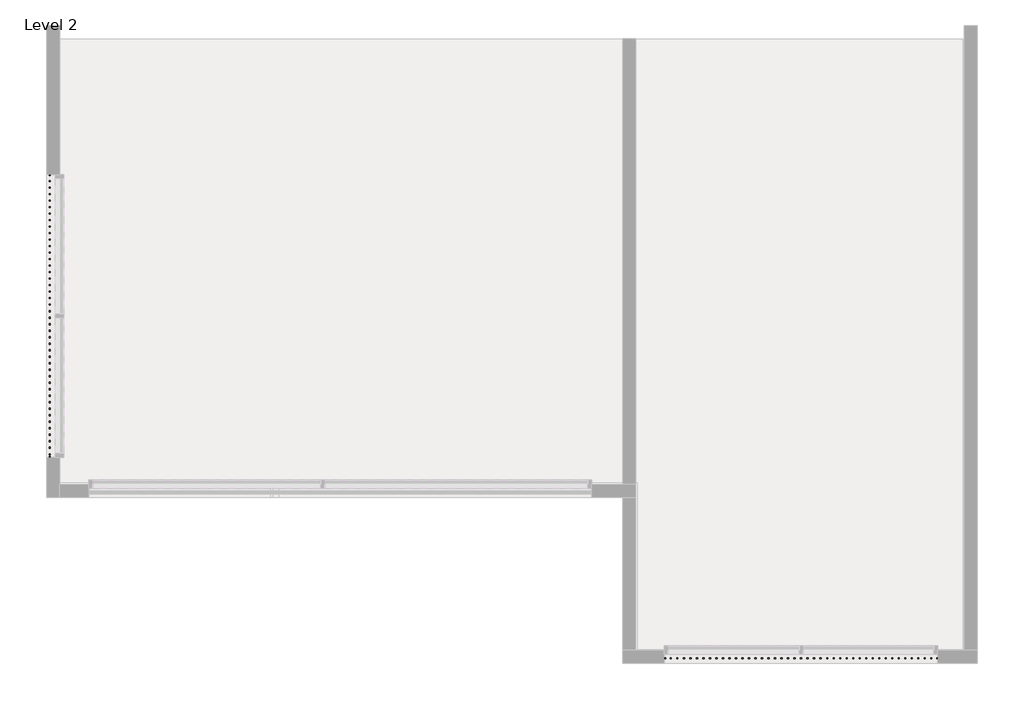
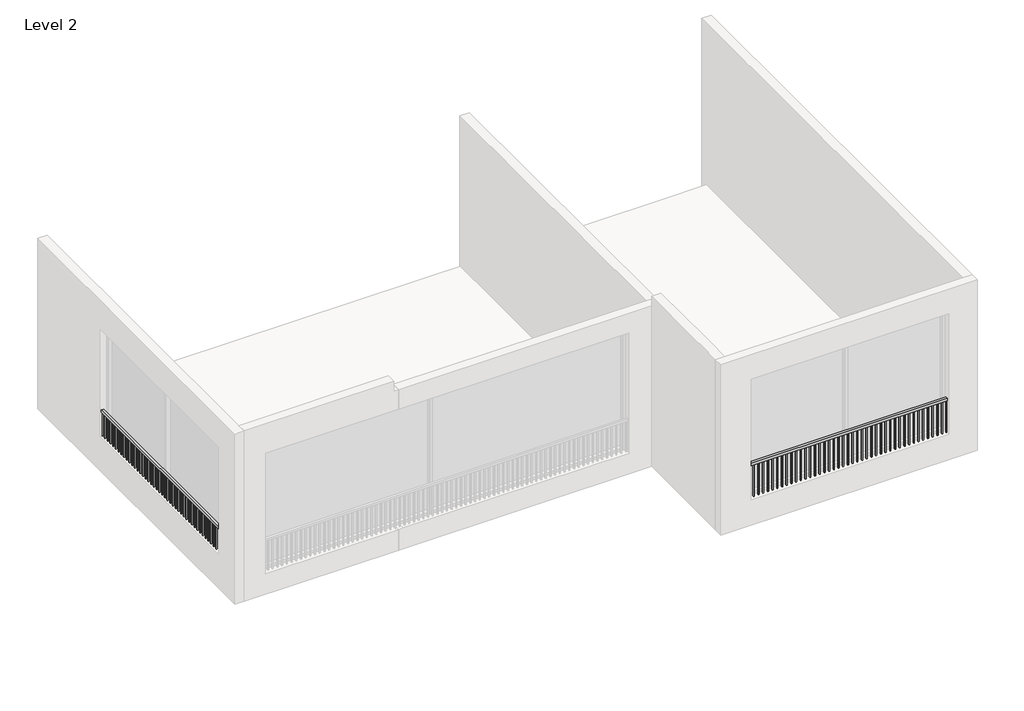
# One storey, part 2 of 2: 2 railings.
"""IFC4 building model written with IfcOpenShell, lengths in millimetres."""

from ifc_helpers import new_model, si_unit, frame, origin, place, context, project, spatial, polyline, outline, extrude, element, save

model = new_model("IFC4")

# Units and contexts
model_context = context("Model", 3, world=origin())
ifc_project = project(units=[si_unit("LENGTHUNIT", "METRE", prefix="MILLI")], contexts=[model_context])

# Site, building, storey
site = spatial("IfcSite", under=ifc_project)
building = spatial("IfcBuilding", under=site)
storey = spatial("IfcBuildingStorey", under=building, Name="Level 2", Elevation=3657.6)

# Railings
placement = place(None, origin())
element("IfcRailing", 1, ObjectType="Handrail - Rectangular", at=placement, inside=storey, context=model_context, shape_type="SweptSolid", body=[
    extrude(outline(polyline([(-6422.5796605, -2958.1874156), (-6422.5796605, -2907.3874156), (-2155.3796605, -2907.3874156), (-2155.3796605, -2958.1874156), (-6422.5796605, -2958.1874156)])), frame((0.0, 0.0, 4978.4), z_axis=(0.0, 0.0, 1.0), x_axis=(1.0, 0.0, 0.0)), (0.0, 0.0, 1.0), 50.8),
    extrude(outline(polyline([(-2266.5046605, -2942.3124156), (-2266.5046605, -2923.2624156), (-2247.4546605, -2923.2624156), (-2247.4546605, -2942.3124156), (-2266.5046605, -2942.3124156)])), frame((0.0, 0.0, 4114.8), z_axis=(0.0, 0.0, 1.0), x_axis=(1.0, 0.0, 0.0)), (0.0, 0.0, 1.0), 863.6),
    extrude(outline(polyline([(-2368.1046605, -2942.3124156), (-2368.1046605, -2923.2624156), (-2349.0546605, -2923.2624156), (-2349.0546605, -2942.3124156), (-2368.1046605, -2942.3124156)])), frame((0.0, 0.0, 4114.8), z_axis=(0.0, 0.0, 1.0), x_axis=(1.0, 0.0, 0.0)), (0.0, 0.0, 1.0), 863.6),
    extrude(outline(polyline([(-2469.7046605, -2942.3124156), (-2469.7046605, -2923.2624156), (-2450.6546605, -2923.2624156), (-2450.6546605, -2942.3124156), (-2469.7046605, -2942.3124156)])), frame((0.0, 0.0, 4114.8), z_axis=(0.0, 0.0, 1.0), x_axis=(1.0, 0.0, 0.0)), (0.0, 0.0, 1.0), 863.6),
    extrude(outline(polyline([(-2571.3046605, -2942.3124156), (-2571.3046605, -2923.2624156), (-2552.2546605, -2923.2624156), (-2552.2546605, -2942.3124156), (-2571.3046605, -2942.3124156)])), frame((0.0, 0.0, 4114.8), z_axis=(0.0, 0.0, 1.0), x_axis=(1.0, 0.0, 0.0)), (0.0, 0.0, 1.0), 863.6),
    extrude(outline(polyline([(-2672.9046605, -2942.3124156), (-2672.9046605, -2923.2624156), (-2653.8546605, -2923.2624156), (-2653.8546605, -2942.3124156), (-2672.9046605, -2942.3124156)])), frame((0.0, 0.0, 4114.8), z_axis=(0.0, 0.0, 1.0), x_axis=(1.0, 0.0, 0.0)), (0.0, 0.0, 1.0), 863.6),
    extrude(outline(polyline([(-2774.5046605, -2942.3124156), (-2774.5046605, -2923.2624156), (-2755.4546605, -2923.2624156), (-2755.4546605, -2942.3124156), (-2774.5046605, -2942.3124156)])), frame((0.0, 0.0, 4114.8), z_axis=(0.0, 0.0, 1.0), x_axis=(1.0, 0.0, 0.0)), (0.0, 0.0, 1.0), 863.6),
    extrude(outline(polyline([(-2876.1046605, -2942.3124156), (-2876.1046605, -2923.2624156), (-2857.0546605, -2923.2624156), (-2857.0546605, -2942.3124156), (-2876.1046605, -2942.3124156)])), frame((0.0, 0.0, 4114.8), z_axis=(0.0, 0.0, 1.0), x_axis=(1.0, 0.0, 0.0)), (0.0, 0.0, 1.0), 863.6),
    extrude(outline(polyline([(-2977.7046605, -2942.3124156), (-2977.7046605, -2923.2624156), (-2958.6546605, -2923.2624156), (-2958.6546605, -2942.3124156), (-2977.7046605, -2942.3124156)])), frame((0.0, 0.0, 4114.8), z_axis=(0.0, 0.0, 1.0), x_axis=(1.0, 0.0, 0.0)), (0.0, 0.0, 1.0), 863.6),
    extrude(outline(polyline([(-3079.3046605, -2942.3124156), (-3079.3046605, -2923.2624156), (-3060.2546605, -2923.2624156), (-3060.2546605, -2942.3124156), (-3079.3046605, -2942.3124156)])), frame((0.0, 0.0, 4114.8), z_axis=(0.0, 0.0, 1.0), x_axis=(1.0, 0.0, 0.0)), (0.0, 0.0, 1.0), 863.6),
    extrude(outline(polyline([(-3180.9046605, -2942.3124156), (-3180.9046605, -2923.2624156), (-3161.8546605, -2923.2624156), (-3161.8546605, -2942.3124156), (-3180.9046605, -2942.3124156)])), frame((0.0, 0.0, 4114.8), z_axis=(0.0, 0.0, 1.0), x_axis=(1.0, 0.0, 0.0)), (0.0, 0.0, 1.0), 863.6),
    extrude(outline(polyline([(-3282.5046605, -2942.3124156), (-3282.5046605, -2923.2624156), (-3263.4546605, -2923.2624156), (-3263.4546605, -2942.3124156), (-3282.5046605, -2942.3124156)])), frame((0.0, 0.0, 4114.8), z_axis=(0.0, 0.0, 1.0), x_axis=(1.0, 0.0, 0.0)), (0.0, 0.0, 1.0), 863.6),
    extrude(outline(polyline([(-3384.1046605, -2942.3124156), (-3384.1046605, -2923.2624156), (-3365.0546605, -2923.2624156), (-3365.0546605, -2942.3124156), (-3384.1046605, -2942.3124156)])), frame((0.0, 0.0, 4114.8), z_axis=(0.0, 0.0, 1.0), x_axis=(1.0, 0.0, 0.0)), (0.0, 0.0, 1.0), 863.6),
    extrude(outline(polyline([(-3485.7046605, -2942.3124156), (-3485.7046605, -2923.2624156), (-3466.6546605, -2923.2624156), (-3466.6546605, -2942.3124156), (-3485.7046605, -2942.3124156)])), frame((0.0, 0.0, 4114.8), z_axis=(0.0, 0.0, 1.0), x_axis=(1.0, 0.0, 0.0)), (0.0, 0.0, 1.0), 863.6),
    extrude(outline(polyline([(-3587.3046605, -2942.3124156), (-3587.3046605, -2923.2624156), (-3568.2546605, -2923.2624156), (-3568.2546605, -2942.3124156), (-3587.3046605, -2942.3124156)])), frame((0.0, 0.0, 4114.8), z_axis=(0.0, 0.0, 1.0), x_axis=(1.0, 0.0, 0.0)), (0.0, 0.0, 1.0), 863.6),
    extrude(outline(polyline([(-3688.9046605, -2942.3124156), (-3688.9046605, -2923.2624156), (-3669.8546605, -2923.2624156), (-3669.8546605, -2942.3124156), (-3688.9046605, -2942.3124156)])), frame((0.0, 0.0, 4114.8), z_axis=(0.0, 0.0, 1.0), x_axis=(1.0, 0.0, 0.0)), (0.0, 0.0, 1.0), 863.6),
    extrude(outline(polyline([(-3790.5046605, -2942.3124156), (-3790.5046605, -2923.2624156), (-3771.4546605, -2923.2624156), (-3771.4546605, -2942.3124156), (-3790.5046605, -2942.3124156)])), frame((0.0, 0.0, 4114.8), z_axis=(0.0, 0.0, 1.0), x_axis=(1.0, 0.0, 0.0)), (0.0, 0.0, 1.0), 863.6),
    extrude(outline(polyline([(-3892.1046605, -2942.3124156), (-3892.1046605, -2923.2624156), (-3873.0546605, -2923.2624156), (-3873.0546605, -2942.3124156), (-3892.1046605, -2942.3124156)])), frame((0.0, 0.0, 4114.8), z_axis=(0.0, 0.0, 1.0), x_axis=(1.0, 0.0, 0.0)), (0.0, 0.0, 1.0), 863.6),
    extrude(outline(polyline([(-3993.7046605, -2942.3124156), (-3993.7046605, -2923.2624156), (-3974.6546605, -2923.2624156), (-3974.6546605, -2942.3124156), (-3993.7046605, -2942.3124156)])), frame((0.0, 0.0, 4114.8), z_axis=(0.0, 0.0, 1.0), x_axis=(1.0, 0.0, 0.0)), (0.0, 0.0, 1.0), 863.6),
    extrude(outline(polyline([(-4095.3046605, -2942.3124156), (-4095.3046605, -2923.2624156), (-4076.2546605, -2923.2624156), (-4076.2546605, -2942.3124156), (-4095.3046605, -2942.3124156)])), frame((0.0, 0.0, 4114.8), z_axis=(0.0, 0.0, 1.0), x_axis=(1.0, 0.0, 0.0)), (0.0, 0.0, 1.0), 863.6),
    extrude(outline(polyline([(-4196.9046605, -2942.3124156), (-4196.9046605, -2923.2624156), (-4177.8546605, -2923.2624156), (-4177.8546605, -2942.3124156), (-4196.9046605, -2942.3124156)])), frame((0.0, 0.0, 4114.8), z_axis=(0.0, 0.0, 1.0), x_axis=(1.0, 0.0, 0.0)), (0.0, 0.0, 1.0), 863.6),
    extrude(outline(polyline([(-4298.5046605, -2942.3124156), (-4298.5046605, -2923.2624156), (-4279.4546605, -2923.2624156), (-4279.4546605, -2942.3124156), (-4298.5046605, -2942.3124156)])), frame((0.0, 0.0, 4114.8), z_axis=(0.0, 0.0, 1.0), x_axis=(1.0, 0.0, 0.0)), (0.0, 0.0, 1.0), 863.6),
    extrude(outline(polyline([(-4400.1046605, -2942.3124156), (-4400.1046605, -2923.2624156), (-4381.0546605, -2923.2624156), (-4381.0546605, -2942.3124156), (-4400.1046605, -2942.3124156)])), frame((0.0, 0.0, 4114.8), z_axis=(0.0, 0.0, 1.0), x_axis=(1.0, 0.0, 0.0)), (0.0, 0.0, 1.0), 863.6),
    extrude(outline(polyline([(-4501.7046605, -2942.3124156), (-4501.7046605, -2923.2624156), (-4482.6546605, -2923.2624156), (-4482.6546605, -2942.3124156), (-4501.7046605, -2942.3124156)])), frame((0.0, 0.0, 4114.8), z_axis=(0.0, 0.0, 1.0), x_axis=(1.0, 0.0, 0.0)), (0.0, 0.0, 1.0), 863.6),
    extrude(outline(polyline([(-4603.3046605, -2942.3124156), (-4603.3046605, -2923.2624156), (-4584.2546605, -2923.2624156), (-4584.2546605, -2942.3124156), (-4603.3046605, -2942.3124156)])), frame((0.0, 0.0, 4114.8), z_axis=(0.0, 0.0, 1.0), x_axis=(1.0, 0.0, 0.0)), (0.0, 0.0, 1.0), 863.6),
    extrude(outline(polyline([(-4704.9046605, -2942.3124156), (-4704.9046605, -2923.2624156), (-4685.8546605, -2923.2624156), (-4685.8546605, -2942.3124156), (-4704.9046605, -2942.3124156)])), frame((0.0, 0.0, 4114.8), z_axis=(0.0, 0.0, 1.0), x_axis=(1.0, 0.0, 0.0)), (0.0, 0.0, 1.0), 863.6),
    extrude(outline(polyline([(-4806.5046605, -2942.3124156), (-4806.5046605, -2923.2624156), (-4787.4546605, -2923.2624156), (-4787.4546605, -2942.3124156), (-4806.5046605, -2942.3124156)])), frame((0.0, 0.0, 4114.8), z_axis=(0.0, 0.0, 1.0), x_axis=(1.0, 0.0, 0.0)), (0.0, 0.0, 1.0), 863.6),
    extrude(outline(polyline([(-4908.1046605, -2942.3124156), (-4908.1046605, -2923.2624156), (-4889.0546605, -2923.2624156), (-4889.0546605, -2942.3124156), (-4908.1046605, -2942.3124156)])), frame((0.0, 0.0, 4114.8), z_axis=(0.0, 0.0, 1.0), x_axis=(1.0, 0.0, 0.0)), (0.0, 0.0, 1.0), 863.6),
    extrude(outline(polyline([(-5009.7046605, -2942.3124156), (-5009.7046605, -2923.2624156), (-4990.6546605, -2923.2624156), (-4990.6546605, -2942.3124156), (-5009.7046605, -2942.3124156)])), frame((0.0, 0.0, 4114.8), z_axis=(0.0, 0.0, 1.0), x_axis=(1.0, 0.0, 0.0)), (0.0, 0.0, 1.0), 863.6),
    extrude(outline(polyline([(-5111.3046605, -2942.3124156), (-5111.3046605, -2923.2624156), (-5092.2546605, -2923.2624156), (-5092.2546605, -2942.3124156), (-5111.3046605, -2942.3124156)])), frame((0.0, 0.0, 4114.8), z_axis=(0.0, 0.0, 1.0), x_axis=(1.0, 0.0, 0.0)), (0.0, 0.0, 1.0), 863.6),
    extrude(outline(polyline([(-5212.9046605, -2942.3124156), (-5212.9046605, -2923.2624156), (-5193.8546605, -2923.2624156), (-5193.8546605, -2942.3124156), (-5212.9046605, -2942.3124156)])), frame((0.0, 0.0, 4114.8), z_axis=(0.0, 0.0, 1.0), x_axis=(1.0, 0.0, 0.0)), (0.0, 0.0, 1.0), 863.6),
    extrude(outline(polyline([(-5314.5046605, -2942.3124156), (-5314.5046605, -2923.2624156), (-5295.4546605, -2923.2624156), (-5295.4546605, -2942.3124156), (-5314.5046605, -2942.3124156)])), frame((0.0, 0.0, 4114.8), z_axis=(0.0, 0.0, 1.0), x_axis=(1.0, 0.0, 0.0)), (0.0, 0.0, 1.0), 863.6),
    extrude(outline(polyline([(-5416.1046605, -2942.3124156), (-5416.1046605, -2923.2624156), (-5397.0546605, -2923.2624156), (-5397.0546605, -2942.3124156), (-5416.1046605, -2942.3124156)])), frame((0.0, 0.0, 4114.8), z_axis=(0.0, 0.0, 1.0), x_axis=(1.0, 0.0, 0.0)), (0.0, 0.0, 1.0), 863.6),
    extrude(outline(polyline([(-5517.7046605, -2942.3124156), (-5517.7046605, -2923.2624156), (-5498.6546605, -2923.2624156), (-5498.6546605, -2942.3124156), (-5517.7046605, -2942.3124156)])), frame((0.0, 0.0, 4114.8), z_axis=(0.0, 0.0, 1.0), x_axis=(1.0, 0.0, 0.0)), (0.0, 0.0, 1.0), 863.6),
    extrude(outline(polyline([(-5619.3046605, -2942.3124156), (-5619.3046605, -2923.2624156), (-5600.2546605, -2923.2624156), (-5600.2546605, -2942.3124156), (-5619.3046605, -2942.3124156)])), frame((0.0, 0.0, 4114.8), z_axis=(0.0, 0.0, 1.0), x_axis=(1.0, 0.0, 0.0)), (0.0, 0.0, 1.0), 863.6),
    extrude(outline(polyline([(-5720.9046605, -2942.3124156), (-5720.9046605, -2923.2624156), (-5701.8546605, -2923.2624156), (-5701.8546605, -2942.3124156), (-5720.9046605, -2942.3124156)])), frame((0.0, 0.0, 4114.8), z_axis=(0.0, 0.0, 1.0), x_axis=(1.0, 0.0, 0.0)), (0.0, 0.0, 1.0), 863.6),
    extrude(outline(polyline([(-5822.5046605, -2942.3124156), (-5822.5046605, -2923.2624156), (-5803.4546605, -2923.2624156), (-5803.4546605, -2942.3124156), (-5822.5046605, -2942.3124156)])), frame((0.0, 0.0, 4114.8), z_axis=(0.0, 0.0, 1.0), x_axis=(1.0, 0.0, 0.0)), (0.0, 0.0, 1.0), 863.6),
    extrude(outline(polyline([(-5924.1046605, -2942.3124156), (-5924.1046605, -2923.2624156), (-5905.0546605, -2923.2624156), (-5905.0546605, -2942.3124156), (-5924.1046605, -2942.3124156)])), frame((0.0, 0.0, 4114.8), z_axis=(0.0, 0.0, 1.0), x_axis=(1.0, 0.0, 0.0)), (0.0, 0.0, 1.0), 863.6),
    extrude(outline(polyline([(-6025.7046605, -2942.3124156), (-6025.7046605, -2923.2624156), (-6006.6546605, -2923.2624156), (-6006.6546605, -2942.3124156), (-6025.7046605, -2942.3124156)])), frame((0.0, 0.0, 4114.8), z_axis=(0.0, 0.0, 1.0), x_axis=(1.0, 0.0, 0.0)), (0.0, 0.0, 1.0), 863.6),
    extrude(outline(polyline([(-6127.3046605, -2942.3124156), (-6127.3046605, -2923.2624156), (-6108.2546605, -2923.2624156), (-6108.2546605, -2942.3124156), (-6127.3046605, -2942.3124156)])), frame((0.0, 0.0, 4114.8), z_axis=(0.0, 0.0, 1.0), x_axis=(1.0, 0.0, 0.0)), (0.0, 0.0, 1.0), 863.6),
    extrude(outline(polyline([(-6228.9046605, -2942.3124156), (-6228.9046605, -2923.2624156), (-6209.8546605, -2923.2624156), (-6209.8546605, -2942.3124156), (-6228.9046605, -2942.3124156)])), frame((0.0, 0.0, 4114.8), z_axis=(0.0, 0.0, 1.0), x_axis=(1.0, 0.0, 0.0)), (0.0, 0.0, 1.0), 863.6),
    extrude(outline(polyline([(-6330.5046605, -2942.3124156), (-6330.5046605, -2923.2624156), (-6311.4546605, -2923.2624156), (-6311.4546605, -2942.3124156), (-6330.5046605, -2942.3124156)])), frame((0.0, 0.0, 4114.8), z_axis=(0.0, 0.0, 1.0), x_axis=(1.0, 0.0, 0.0)), (0.0, 0.0, 1.0), 863.6),
    extrude(outline(polyline([(-2174.4296605, -2942.3124156), (-2174.4296605, -2923.2624156), (-2155.3796605, -2923.2624156), (-2155.3796605, -2942.3124156), (-2174.4296605, -2942.3124156)])), frame((0.0, 0.0, 4114.8), z_axis=(0.0, 0.0, 1.0), x_axis=(1.0, 0.0, 0.0)), (0.0, 0.0, 1.0), 863.6),
    extrude(outline(polyline([(-6422.5796605, -2942.3124156), (-6422.5796605, -2923.2624156), (-6403.5296605, -2923.2624156), (-6403.5296605, -2942.3124156), (-6422.5796605, -2942.3124156)])), frame((0.0, 0.0, 4114.8), z_axis=(0.0, 0.0, 1.0), x_axis=(1.0, 0.0, 0.0)), (0.0, 0.0, 1.0), 863.6),
])
element("IfcRailing", 2, ObjectType="Handrail - Rectangular", at=placement, inside=storey, context=model_context, shape_type="SweptSolid", body=[
    extrude(outline(polyline([(-16039.6141623, 4621.1544753), (-15988.8141623, 4621.1544753), (-15988.8141623, 201.5544753), (-16039.6141623, 201.5544753), (-16039.6141623, 4621.1544753)])), frame((0.0, 0.0, 4978.4), z_axis=(0.0, 0.0, 1.0), x_axis=(1.0, 0.0, 0.0)), (0.0, 0.0, 1.0), 50.8),
    extrude(outline(polyline([(-16023.7391623, 261.8794753), (-16004.6891623, 261.8794753), (-16004.6891623, 242.8294753), (-16023.7391623, 242.8294753), (-16023.7391623, 261.8794753)])), frame((0.0, 0.0, 4114.8), z_axis=(0.0, 0.0, 1.0), x_axis=(1.0, 0.0, 0.0)), (0.0, 0.0, 1.0), 863.6),
    extrude(outline(polyline([(-16023.7391623, 363.4794753), (-16004.6891623, 363.4794753), (-16004.6891623, 344.4294753), (-16023.7391623, 344.4294753), (-16023.7391623, 363.4794753)])), frame((0.0, 0.0, 4114.8), z_axis=(0.0, 0.0, 1.0), x_axis=(1.0, 0.0, 0.0)), (0.0, 0.0, 1.0), 863.6),
    extrude(outline(polyline([(-16023.7391623, 465.0794753), (-16004.6891623, 465.0794753), (-16004.6891623, 446.0294753), (-16023.7391623, 446.0294753), (-16023.7391623, 465.0794753)])), frame((0.0, 0.0, 4114.8), z_axis=(0.0, 0.0, 1.0), x_axis=(1.0, 0.0, 0.0)), (0.0, 0.0, 1.0), 863.6),
    extrude(outline(polyline([(-16023.7391623, 566.6794753), (-16004.6891623, 566.6794753), (-16004.6891623, 547.6294753), (-16023.7391623, 547.6294753), (-16023.7391623, 566.6794753)])), frame((0.0, 0.0, 4114.8), z_axis=(0.0, 0.0, 1.0), x_axis=(1.0, 0.0, 0.0)), (0.0, 0.0, 1.0), 863.6),
    extrude(outline(polyline([(-16023.7391623, 668.2794753), (-16004.6891623, 668.2794753), (-16004.6891623, 649.2294753), (-16023.7391623, 649.2294753), (-16023.7391623, 668.2794753)])), frame((0.0, 0.0, 4114.8), z_axis=(0.0, 0.0, 1.0), x_axis=(1.0, 0.0, 0.0)), (0.0, 0.0, 1.0), 863.6),
    extrude(outline(polyline([(-16023.7391623, 769.8794753), (-16004.6891623, 769.8794753), (-16004.6891623, 750.8294753), (-16023.7391623, 750.8294753), (-16023.7391623, 769.8794753)])), frame((0.0, 0.0, 4114.8), z_axis=(0.0, 0.0, 1.0), x_axis=(1.0, 0.0, 0.0)), (0.0, 0.0, 1.0), 863.6),
    extrude(outline(polyline([(-16023.7391623, 871.4794753), (-16004.6891623, 871.4794753), (-16004.6891623, 852.4294753), (-16023.7391623, 852.4294753), (-16023.7391623, 871.4794753)])), frame((0.0, 0.0, 4114.8), z_axis=(0.0, 0.0, 1.0), x_axis=(1.0, 0.0, 0.0)), (0.0, 0.0, 1.0), 863.6),
    extrude(outline(polyline([(-16023.7391623, 973.0794753), (-16004.6891623, 973.0794753), (-16004.6891623, 954.0294753), (-16023.7391623, 954.0294753), (-16023.7391623, 973.0794753)])), frame((0.0, 0.0, 4114.8), z_axis=(0.0, 0.0, 1.0), x_axis=(1.0, 0.0, 0.0)), (0.0, 0.0, 1.0), 863.6),
    extrude(outline(polyline([(-16023.7391623, 1074.6794753), (-16004.6891623, 1074.6794753), (-16004.6891623, 1055.6294753), (-16023.7391623, 1055.6294753), (-16023.7391623, 1074.6794753)])), frame((0.0, 0.0, 4114.8), z_axis=(0.0, 0.0, 1.0), x_axis=(1.0, 0.0, 0.0)), (0.0, 0.0, 1.0), 863.6),
    extrude(outline(polyline([(-16023.7391623, 1176.2794753), (-16004.6891623, 1176.2794753), (-16004.6891623, 1157.2294753), (-16023.7391623, 1157.2294753), (-16023.7391623, 1176.2794753)])), frame((0.0, 0.0, 4114.8), z_axis=(0.0, 0.0, 1.0), x_axis=(1.0, 0.0, 0.0)), (0.0, 0.0, 1.0), 863.6),
    extrude(outline(polyline([(-16023.7391623, 1277.8794753), (-16004.6891623, 1277.8794753), (-16004.6891623, 1258.8294753), (-16023.7391623, 1258.8294753), (-16023.7391623, 1277.8794753)])), frame((0.0, 0.0, 4114.8), z_axis=(0.0, 0.0, 1.0), x_axis=(1.0, 0.0, 0.0)), (0.0, 0.0, 1.0), 863.6),
    extrude(outline(polyline([(-16023.7391623, 1379.4794753), (-16004.6891623, 1379.4794753), (-16004.6891623, 1360.4294753), (-16023.7391623, 1360.4294753), (-16023.7391623, 1379.4794753)])), frame((0.0, 0.0, 4114.8), z_axis=(0.0, 0.0, 1.0), x_axis=(1.0, 0.0, 0.0)), (0.0, 0.0, 1.0), 863.6),
    extrude(outline(polyline([(-16023.7391623, 1481.0794753), (-16004.6891623, 1481.0794753), (-16004.6891623, 1462.0294753), (-16023.7391623, 1462.0294753), (-16023.7391623, 1481.0794753)])), frame((0.0, 0.0, 4114.8), z_axis=(0.0, 0.0, 1.0), x_axis=(1.0, 0.0, 0.0)), (0.0, 0.0, 1.0), 863.6),
    extrude(outline(polyline([(-16023.7391623, 1582.6794753), (-16004.6891623, 1582.6794753), (-16004.6891623, 1563.6294753), (-16023.7391623, 1563.6294753), (-16023.7391623, 1582.6794753)])), frame((0.0, 0.0, 4114.8), z_axis=(0.0, 0.0, 1.0), x_axis=(1.0, 0.0, 0.0)), (0.0, 0.0, 1.0), 863.6),
    extrude(outline(polyline([(-16023.7391623, 1684.2794753), (-16004.6891623, 1684.2794753), (-16004.6891623, 1665.2294753), (-16023.7391623, 1665.2294753), (-16023.7391623, 1684.2794753)])), frame((0.0, 0.0, 4114.8), z_axis=(0.0, 0.0, 1.0), x_axis=(1.0, 0.0, 0.0)), (0.0, 0.0, 1.0), 863.6),
    extrude(outline(polyline([(-16023.7391623, 1785.8794753), (-16004.6891623, 1785.8794753), (-16004.6891623, 1766.8294753), (-16023.7391623, 1766.8294753), (-16023.7391623, 1785.8794753)])), frame((0.0, 0.0, 4114.8), z_axis=(0.0, 0.0, 1.0), x_axis=(1.0, 0.0, 0.0)), (0.0, 0.0, 1.0), 863.6),
    extrude(outline(polyline([(-16023.7391623, 1887.4794753), (-16004.6891623, 1887.4794753), (-16004.6891623, 1868.4294753), (-16023.7391623, 1868.4294753), (-16023.7391623, 1887.4794753)])), frame((0.0, 0.0, 4114.8), z_axis=(0.0, 0.0, 1.0), x_axis=(1.0, 0.0, 0.0)), (0.0, 0.0, 1.0), 863.6),
    extrude(outline(polyline([(-16023.7391623, 1989.0794753), (-16004.6891623, 1989.0794753), (-16004.6891623, 1970.0294753), (-16023.7391623, 1970.0294753), (-16023.7391623, 1989.0794753)])), frame((0.0, 0.0, 4114.8), z_axis=(0.0, 0.0, 1.0), x_axis=(1.0, 0.0, 0.0)), (0.0, 0.0, 1.0), 863.6),
    extrude(outline(polyline([(-16023.7391623, 2090.6794753), (-16004.6891623, 2090.6794753), (-16004.6891623, 2071.6294753), (-16023.7391623, 2071.6294753), (-16023.7391623, 2090.6794753)])), frame((0.0, 0.0, 4114.8), z_axis=(0.0, 0.0, 1.0), x_axis=(1.0, 0.0, 0.0)), (0.0, 0.0, 1.0), 863.6),
    extrude(outline(polyline([(-16023.7391623, 2192.2794753), (-16004.6891623, 2192.2794753), (-16004.6891623, 2173.2294753), (-16023.7391623, 2173.2294753), (-16023.7391623, 2192.2794753)])), frame((0.0, 0.0, 4114.8), z_axis=(0.0, 0.0, 1.0), x_axis=(1.0, 0.0, 0.0)), (0.0, 0.0, 1.0), 863.6),
    extrude(outline(polyline([(-16023.7391623, 2293.8794753), (-16004.6891623, 2293.8794753), (-16004.6891623, 2274.8294753), (-16023.7391623, 2274.8294753), (-16023.7391623, 2293.8794753)])), frame((0.0, 0.0, 4114.8), z_axis=(0.0, 0.0, 1.0), x_axis=(1.0, 0.0, 0.0)), (0.0, 0.0, 1.0), 863.6),
    extrude(outline(polyline([(-16023.7391623, 2395.4794753), (-16004.6891623, 2395.4794753), (-16004.6891623, 2376.4294753), (-16023.7391623, 2376.4294753), (-16023.7391623, 2395.4794753)])), frame((0.0, 0.0, 4114.8), z_axis=(0.0, 0.0, 1.0), x_axis=(1.0, 0.0, 0.0)), (0.0, 0.0, 1.0), 863.6),
    extrude(outline(polyline([(-16023.7391623, 2497.0794753), (-16004.6891623, 2497.0794753), (-16004.6891623, 2478.0294753), (-16023.7391623, 2478.0294753), (-16023.7391623, 2497.0794753)])), frame((0.0, 0.0, 4114.8), z_axis=(0.0, 0.0, 1.0), x_axis=(1.0, 0.0, 0.0)), (0.0, 0.0, 1.0), 863.6),
    extrude(outline(polyline([(-16023.7391623, 2598.6794753), (-16004.6891623, 2598.6794753), (-16004.6891623, 2579.6294753), (-16023.7391623, 2579.6294753), (-16023.7391623, 2598.6794753)])), frame((0.0, 0.0, 4114.8), z_axis=(0.0, 0.0, 1.0), x_axis=(1.0, 0.0, 0.0)), (0.0, 0.0, 1.0), 863.6),
    extrude(outline(polyline([(-16023.7391623, 2700.2794753), (-16004.6891623, 2700.2794753), (-16004.6891623, 2681.2294753), (-16023.7391623, 2681.2294753), (-16023.7391623, 2700.2794753)])), frame((0.0, 0.0, 4114.8), z_axis=(0.0, 0.0, 1.0), x_axis=(1.0, 0.0, 0.0)), (0.0, 0.0, 1.0), 863.6),
    extrude(outline(polyline([(-16023.7391623, 2801.8794753), (-16004.6891623, 2801.8794753), (-16004.6891623, 2782.8294753), (-16023.7391623, 2782.8294753), (-16023.7391623, 2801.8794753)])), frame((0.0, 0.0, 4114.8), z_axis=(0.0, 0.0, 1.0), x_axis=(1.0, 0.0, 0.0)), (0.0, 0.0, 1.0), 863.6),
    extrude(outline(polyline([(-16023.7391623, 2903.4794753), (-16004.6891623, 2903.4794753), (-16004.6891623, 2884.4294753), (-16023.7391623, 2884.4294753), (-16023.7391623, 2903.4794753)])), frame((0.0, 0.0, 4114.8), z_axis=(0.0, 0.0, 1.0), x_axis=(1.0, 0.0, 0.0)), (0.0, 0.0, 1.0), 863.6),
    extrude(outline(polyline([(-16023.7391623, 3005.0794753), (-16004.6891623, 3005.0794753), (-16004.6891623, 2986.0294753), (-16023.7391623, 2986.0294753), (-16023.7391623, 3005.0794753)])), frame((0.0, 0.0, 4114.8), z_axis=(0.0, 0.0, 1.0), x_axis=(1.0, 0.0, 0.0)), (0.0, 0.0, 1.0), 863.6),
    extrude(outline(polyline([(-16023.7391623, 3106.6794753), (-16004.6891623, 3106.6794753), (-16004.6891623, 3087.6294753), (-16023.7391623, 3087.6294753), (-16023.7391623, 3106.6794753)])), frame((0.0, 0.0, 4114.8), z_axis=(0.0, 0.0, 1.0), x_axis=(1.0, 0.0, 0.0)), (0.0, 0.0, 1.0), 863.6),
    extrude(outline(polyline([(-16023.7391623, 3208.2794753), (-16004.6891623, 3208.2794753), (-16004.6891623, 3189.2294753), (-16023.7391623, 3189.2294753), (-16023.7391623, 3208.2794753)])), frame((0.0, 0.0, 4114.8), z_axis=(0.0, 0.0, 1.0), x_axis=(1.0, 0.0, 0.0)), (0.0, 0.0, 1.0), 863.6),
    extrude(outline(polyline([(-16023.7391623, 3309.8794753), (-16004.6891623, 3309.8794753), (-16004.6891623, 3290.8294753), (-16023.7391623, 3290.8294753), (-16023.7391623, 3309.8794753)])), frame((0.0, 0.0, 4114.8), z_axis=(0.0, 0.0, 1.0), x_axis=(1.0, 0.0, 0.0)), (0.0, 0.0, 1.0), 863.6),
    extrude(outline(polyline([(-16023.7391623, 3411.4794753), (-16004.6891623, 3411.4794753), (-16004.6891623, 3392.4294753), (-16023.7391623, 3392.4294753), (-16023.7391623, 3411.4794753)])), frame((0.0, 0.0, 4114.8), z_axis=(0.0, 0.0, 1.0), x_axis=(1.0, 0.0, 0.0)), (0.0, 0.0, 1.0), 863.6),
    extrude(outline(polyline([(-16023.7391623, 3513.0794753), (-16004.6891623, 3513.0794753), (-16004.6891623, 3494.0294753), (-16023.7391623, 3494.0294753), (-16023.7391623, 3513.0794753)])), frame((0.0, 0.0, 4114.8), z_axis=(0.0, 0.0, 1.0), x_axis=(1.0, 0.0, 0.0)), (0.0, 0.0, 1.0), 863.6),
    extrude(outline(polyline([(-16023.7391623, 3614.6794753), (-16004.6891623, 3614.6794753), (-16004.6891623, 3595.6294753), (-16023.7391623, 3595.6294753), (-16023.7391623, 3614.6794753)])), frame((0.0, 0.0, 4114.8), z_axis=(0.0, 0.0, 1.0), x_axis=(1.0, 0.0, 0.0)), (0.0, 0.0, 1.0), 863.6),
    extrude(outline(polyline([(-16023.7391623, 3716.2794753), (-16004.6891623, 3716.2794753), (-16004.6891623, 3697.2294753), (-16023.7391623, 3697.2294753), (-16023.7391623, 3716.2794753)])), frame((0.0, 0.0, 4114.8), z_axis=(0.0, 0.0, 1.0), x_axis=(1.0, 0.0, 0.0)), (0.0, 0.0, 1.0), 863.6),
    extrude(outline(polyline([(-16023.7391623, 3817.8794753), (-16004.6891623, 3817.8794753), (-16004.6891623, 3798.8294753), (-16023.7391623, 3798.8294753), (-16023.7391623, 3817.8794753)])), frame((0.0, 0.0, 4114.8), z_axis=(0.0, 0.0, 1.0), x_axis=(1.0, 0.0, 0.0)), (0.0, 0.0, 1.0), 863.6),
    extrude(outline(polyline([(-16023.7391623, 3919.4794753), (-16004.6891623, 3919.4794753), (-16004.6891623, 3900.4294753), (-16023.7391623, 3900.4294753), (-16023.7391623, 3919.4794753)])), frame((0.0, 0.0, 4114.8), z_axis=(0.0, 0.0, 1.0), x_axis=(1.0, 0.0, 0.0)), (0.0, 0.0, 1.0), 863.6),
    extrude(outline(polyline([(-16023.7391623, 4021.0794753), (-16004.6891623, 4021.0794753), (-16004.6891623, 4002.0294753), (-16023.7391623, 4002.0294753), (-16023.7391623, 4021.0794753)])), frame((0.0, 0.0, 4114.8), z_axis=(0.0, 0.0, 1.0), x_axis=(1.0, 0.0, 0.0)), (0.0, 0.0, 1.0), 863.6),
    extrude(outline(polyline([(-16023.7391623, 4122.6794753), (-16004.6891623, 4122.6794753), (-16004.6891623, 4103.6294753), (-16023.7391623, 4103.6294753), (-16023.7391623, 4122.6794753)])), frame((0.0, 0.0, 4114.8), z_axis=(0.0, 0.0, 1.0), x_axis=(1.0, 0.0, 0.0)), (0.0, 0.0, 1.0), 863.6),
    extrude(outline(polyline([(-16023.7391623, 4224.2794753), (-16004.6891623, 4224.2794753), (-16004.6891623, 4205.2294753), (-16023.7391623, 4205.2294753), (-16023.7391623, 4224.2794753)])), frame((0.0, 0.0, 4114.8), z_axis=(0.0, 0.0, 1.0), x_axis=(1.0, 0.0, 0.0)), (0.0, 0.0, 1.0), 863.6),
    extrude(outline(polyline([(-16023.7391623, 4325.8794753), (-16004.6891623, 4325.8794753), (-16004.6891623, 4306.8294753), (-16023.7391623, 4306.8294753), (-16023.7391623, 4325.8794753)])), frame((0.0, 0.0, 4114.8), z_axis=(0.0, 0.0, 1.0), x_axis=(1.0, 0.0, 0.0)), (0.0, 0.0, 1.0), 863.6),
    extrude(outline(polyline([(-16023.7391623, 4427.4794753), (-16004.6891623, 4427.4794753), (-16004.6891623, 4408.4294753), (-16023.7391623, 4408.4294753), (-16023.7391623, 4427.4794753)])), frame((0.0, 0.0, 4114.8), z_axis=(0.0, 0.0, 1.0), x_axis=(1.0, 0.0, 0.0)), (0.0, 0.0, 1.0), 863.6),
    extrude(outline(polyline([(-16023.7391623, 4529.0794753), (-16004.6891623, 4529.0794753), (-16004.6891623, 4510.0294753), (-16023.7391623, 4510.0294753), (-16023.7391623, 4529.0794753)])), frame((0.0, 0.0, 4114.8), z_axis=(0.0, 0.0, 1.0), x_axis=(1.0, 0.0, 0.0)), (0.0, 0.0, 1.0), 863.6),
    extrude(outline(polyline([(-16023.7391623, 220.6044753), (-16004.6891623, 220.6044753), (-16004.6891623, 201.5544753), (-16023.7391623, 201.5544753), (-16023.7391623, 220.6044753)])), frame((0.0, 0.0, 4114.8), z_axis=(0.0, 0.0, 1.0), x_axis=(1.0, 0.0, 0.0)), (0.0, 0.0, 1.0), 863.6),
    extrude(outline(polyline([(-16023.7391623, 4621.1544753), (-16004.6891623, 4621.1544753), (-16004.6891623, 4602.1044753), (-16023.7391623, 4602.1044753), (-16023.7391623, 4621.1544753)])), frame((0.0, 0.0, 4114.8), z_axis=(0.0, 0.0, 1.0), x_axis=(1.0, 0.0, 0.0)), (0.0, 0.0, 1.0), 863.6),
])

save(model, "model.ifc")

# Revit data of these elements
# Type "Handrail - Rectangular"
#   Assembly Code = "C2010400"
#   built-in parameter 1008612 = 0.0416667 (stored number, unit not read)
#   built-in parameter 1008611 = 0.0416667 (stored number, unit not read)
#   built-in parameter 1008609 = 0.333333 (stored number, unit not read)
#   built-in parameter 1008604 = 0.166667 (stored number, unit not read)
#   built-in parameter 1008603 = 0.166667 (stored number, unit not read)
#   Railing Height = 3' - 0"
#   built-in parameter 1008630 = 2
#   built-in parameter 1008610 = 2
#   built-in parameter 1008618 = Baluster - Square : 3/4"
# Elements 1, 2 (IfcRailing, "Handrail - Rectangular")
#   built-in parameter 1008621 = 1.5 (stored number, unit not read)
#   Phase Created = New Construction
